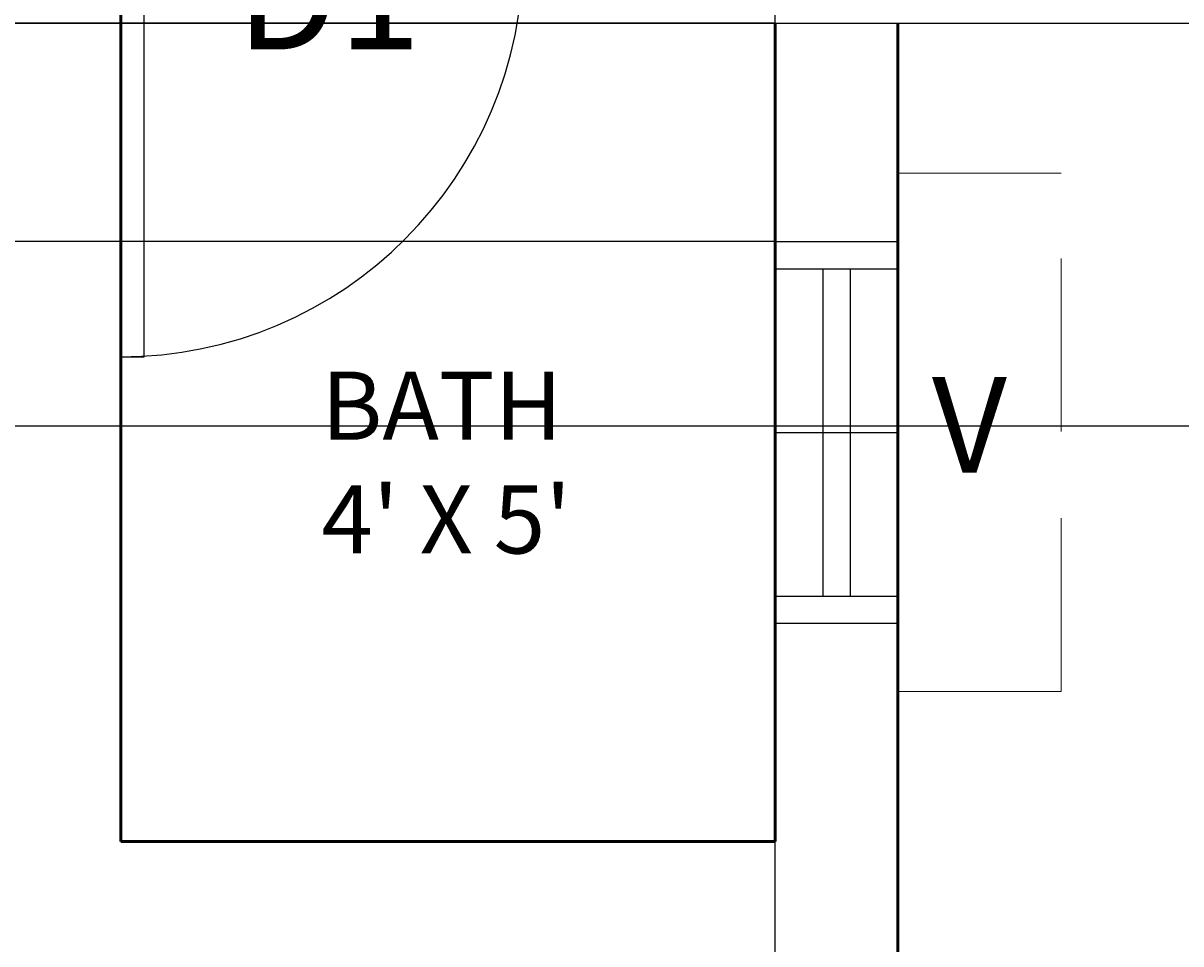
# Model space of a CAD drawing. Units: inches. Extents: x 37 to 824, y -700 to 234.
# Tile 67 of 77: x 364 to 449, y 8 to 75. Entities that reach past the tile are written whole.
import ezdxf

# ---------------------------------------------------------------- set-up
doc = ezdxf.new("R2010")
doc.units = ezdxf.units.IN
doc.header["$MEASUREMENT"] = 0
doc.linetypes.add('DASHED', pattern=[19.05, 12.7, -6.35])
for name, color, linetype, lineweight in [('A-ANNO-DIMS', 2, 'Continuous', 18), ('A-ANNO-TEXT', 7, 'Continuous', 18), ('A-AREA-IDEN', 3, 'Continuous', 18), ('A-DOOR', 4, 'Continuous', 25), ('A-GLAZ', 4, 'Continuous', 25), ('A-ROOF-OVHD', 1, 'DASHED', 18), ('A-WALL', 2, 'Continuous', 50)]:
    doc.layers.add(name, color=color, linetype=linetype, lineweight=lineweight)
doc.styles.get("Standard").update_dxf_attribs({"font": 'arial.ttf'})
doc.dimstyles.get("Standard").update_dxf_attribs({"dimtxt": 0.18, "dimasz": 0.18, "dimexe": 0.18, "dimexo": 0.0625, "dimgap": 0.09, "dimtad": 0, "dimtih": 1, "dimtoh": 1, "dimdec": 1, "dimzin": 0, "dimdsep": 46, "dimlunit": 4, "dimtxsty": 'Standard', "dimcen": 0.09, "dimadec": 0, "dimazin": 0, "dimtfac": 1, "dimtdec": 1, "dimtofl": 0, "dimtmove": 0, "dimatfit": 3, "dimfxl": 1, "dimtolj": 1, "dimtzin": 0, "dimarcsym": 0})

# ---------------------------------------------------------------- blocks, each defined once
blk = doc.blocks.new('*U6')
for p, q in [((-750, 0), (-750, -100)), ((0, 0), (0, -100))]:
    blk.add_line(p, q)
blk.add_lwpolyline([(0, 0), (0, 750), (-43.75, 750), (-43.75, 0)], close=True)
blk.add_arc((0, 0), 750, 90, 180)
blk = doc.blocks.new('VENT-600')
for p, q in [((0, 28), (9, 28)), ((0, 26), (9, 26)), ((3.5, 26), (3.5, 2)), ((5.5, 26), (5.5, 2)), ((0, 14), (9, 14)), ((0, 2), (9, 2)), ((0, 0), (9, 0))]:
    blk.add_line(p, q)
blk = doc.blocks.new('*D61')
at = {"layer": 'A-ANNO-DIMS', "color": 0, "lineweight": -2, "ltscale": 0.5, "transparency": 16777216}
for p, q in [((419.015, 75.09), (78.159, 75.09)), ((78.339, 74.91), (78.339, 67.271)), ((78.339, 59.27), (78.339, 66.91)), ((419.015, 59.09), (78.159, 59.09))]:
    blk.add_line(p, q, dxfattribs=at)
at = {"layer": 'A-ANNO-DIMS', "color": 0, "ltscale": 0.5, "transparency": 16777216}
for points in [[(78.309, 74.91), (78.369, 74.91), (78.339, 75.09)], [(78.309, 59.27), (78.369, 59.27), (78.339, 59.09)]]:
    blk.add_solid(points, dxfattribs=at)
at = {"layer": 'Defpoints', "color": 0, "ltscale": 0.5, "transparency": 16777216}
for p in [(419.077, 75.09), (78.339, 59.09), (419.077, 59.09)]:
    blk.add_point(p, dxfattribs=at)
at = {"layer": 'A-ANNO-DIMS', "color": 0, "ltscale": 0.5, "transparency": 16777216, "insert": (78.339, 67.09), "char_height": 0.18, "attachment_point": 5}
blk.add_mtext('\\A1;1\'-4"', dxfattribs=at)
blk = doc.blocks.new('*D64')
at = {"layer": 'A-ANNO-DIMS', "color": 0, "lineweight": -2, "ltscale": 0.5, "transparency": 16777216}
for p, q in [((428.14, 191.09), (513.773, 191.09)), ((513.593, 190.91), (513.593, -87.228)), ((513.593, -365.73), (513.593, -87.591)), ((428.14, -365.91), (513.773, -365.91))]:
    blk.add_line(p, q, dxfattribs=at)
at = {"layer": 'A-ANNO-DIMS', "color": 0, "ltscale": 0.5, "transparency": 16777216}
for points in [[(513.563, 190.91), (513.623, 190.91), (513.593, 191.09)], [(513.563, -365.73), (513.623, -365.73), (513.593, -365.91)]]:
    blk.add_solid(points, dxfattribs=at)
at = {"layer": 'Defpoints', "color": 0, "ltscale": 0.5, "transparency": 16777216}
for p in [(428.077, 191.09), (428.077, -365.91), (513.593, -365.91)]:
    blk.add_point(p, dxfattribs=at)
at = {"layer": 'A-ANNO-DIMS', "color": 0, "ltscale": 0.5, "transparency": 16777216, "insert": (513.593, -87.41), "char_height": 0.18, "attachment_point": 5}
blk.add_mtext('\\A1;46\'-5"', dxfattribs=at)
blk = doc.blocks.new('*D76')
at = {"layer": 'A-ANNO-DIMS', "color": 0, "lineweight": -2, "ltscale": 0.5, "transparency": 16777216}
for p, q in [((227.14, 75.09), (513.773, 75.09)), ((513.593, 74.91), (513.593, 60.51)), ((513.593, 45.743), (513.593, 60.144)), ((227.14, 45.563), (513.773, 45.563))]:
    blk.add_line(p, q, dxfattribs=at)
at = {"layer": 'A-ANNO-DIMS', "color": 0, "ltscale": 0.5, "transparency": 16777216}
for points in [[(513.563, 74.91), (513.623, 74.91), (513.593, 75.09)], [(513.563, 45.743), (513.623, 45.743), (513.593, 45.563)]]:
    blk.add_solid(points, dxfattribs=at)
at = {"layer": 'Defpoints', "color": 0, "ltscale": 0.5, "transparency": 16777216}
for p in [(227.077, 75.09), (227.077, 45.563), (513.593, 45.563)]:
    blk.add_point(p, dxfattribs=at)
at = {"layer": 'A-ANNO-DIMS', "color": 0, "ltscale": 0.5, "transparency": 16777216, "insert": (513.593, 60.327), "char_height": 0.18, "attachment_point": 5}
blk.add_mtext('\\A1;2\'-5 1/2"', dxfattribs=at)
blk = doc.blocks.new('*D83')
at = {"layer": 'A-ANNO-DIMS', "color": 0, "lineweight": -2, "ltscale": 0.5, "transparency": 16777216}
for p, q in [((358.132, -206.847), (358.132, 234.17)), ((358.312, 233.99), (388.275, 233.99)), ((418.897, 233.99), (388.934, 233.99)), ((419.077, -206.847), (419.077, 234.17))]:
    blk.add_line(p, q, dxfattribs=at)
at = {"layer": 'A-ANNO-DIMS', "color": 0, "ltscale": 0.5, "transparency": 16777216}
for points in [[(358.312, 234.02), (358.312, 233.96), (358.132, 233.99)], [(418.897, 234.02), (418.897, 233.96), (419.077, 233.99)]]:
    blk.add_solid(points, dxfattribs=at)
at = {"layer": 'Defpoints', "color": 0, "ltscale": 0.5, "transparency": 16777216}
for p in [(419.077, 233.99), (358.132, -206.91), (419.077, -206.91)]:
    blk.add_point(p, dxfattribs=at)
at = {"layer": 'A-ANNO-DIMS', "color": 0, "ltscale": 0.5, "transparency": 16777216, "insert": (388.605, 233.99), "char_height": 0.18, "attachment_point": 5}
blk.add_mtext('\\A1;5\'-1"', dxfattribs=at)

msp = doc.modelspace()

# ---------------------------------------------------------------- linework, layer by layer
at = {"layer": 'A-ROOF-OVHD'}
for p, q in [((428.077, 59.09), (428.077, 64.09)), ((428.077, 64.09), (440.077, 64.09)), ((440.077, 26.09), (440.077, 64.09)), ((428.077, 31.09), (428.077, 26.09)), ((428.077, 26.09), (440.077, 26.09))]:
    msp.add_line(p, q, dxfattribs=at)
at = {"layer": 'A-WALL'}
for p, q in [((371.077, 15.09), (371.077, 84.09)), ((419.077, 75.09), (419.077, 15.09)), ((428.077, 75.09), (428.077, 6.09)), ((419.077, 15.09), (371.077, 15.09)), ((419.077, 15.09), (371.077, 15.09))]:
    msp.add_line(p, q, dxfattribs=at)

# ---------------------------------------------------------------- block references
at = {"layer": 'A-DOOR', "xscale": 0.0393700787401575, "yscale": 0.0393700787401575, "zscale": 0.0393700787401575, "rotation": 180}
msp.add_blockref('*U6', (371.077, 80.153), dxfattribs=at)
at = {"layer": 'A-GLAZ'}
msp.add_blockref('VENT-600', (419.077, 31.09), dxfattribs=at)

# ---------------------------------------------------------------- texts
at = {"layer": 'A-ANNO-TEXT'}
for s, height, p in [('D1', 8, (379.536, 73.162)), ('V', 7, (430.587, 42.139))]:
    msp.add_text(s, height=height, dxfattribs=at).set_placement(p)
at = {"layer": 'A-AREA-IDEN', "insert": (381.21, 49.542), "char_height": 5, "attachment_point": 1}
msp.add_mtext_dynamic_manual_height_columns("   BATH\\P   4' X 5'", width=88.32168, gutter_width=1, heights=[0], dxfattribs=at)

# ---------------------------------------------------------------- dimensions: what is measured, and where the dimension line sits
at = {"layer": 'A-ANNO-DIMS', "ltscale": 0.5}
dim = msp.add_linear_dim(base=(419.077, 233.99), p1=(358.132, -206.91), p2=(419.077, -206.91), dimstyle='Standard', override={"dimdec": 1, "dimlfac": 1, "dimrnd": 0, "dimzin": 1, "dimdsep": 46, "dimlunit": 4, "dimfrac": 2}, dxfattribs=at)
dim.commit()
dim.dimension.update_dxf_attribs({"geometry": '*D83', "text_midpoint": (388.605, 233.99)})
for base, p1, p2, picture, middle in [((513.593, -365.91), (428.077, 191.09), (428.077, -365.91), '*D64', (513.593, -87.41)), ((78.339, 59.09), (419.077, 75.09), (419.077, 59.09), '*D61', (78.339, 67.09)), ((513.593, 45.563), (227.077, 75.09), (227.077, 45.563), '*D76', (513.593, 60.327))]:
    dim = msp.add_linear_dim(base=base, p1=p1, p2=p2, angle=90, dimstyle='Standard', override={"dimdec": 1, "dimlfac": 1, "dimrnd": 0, "dimzin": 1, "dimdsep": 46, "dimlunit": 4, "dimfrac": 2}, dxfattribs=at)
    dim.commit()
    dim.dimension.update_dxf_attribs({"geometry": picture, "text_midpoint": middle})

doc.saveas('drawing.dxf')
